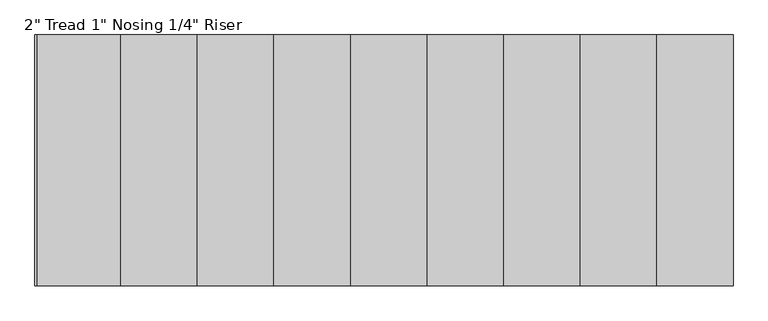
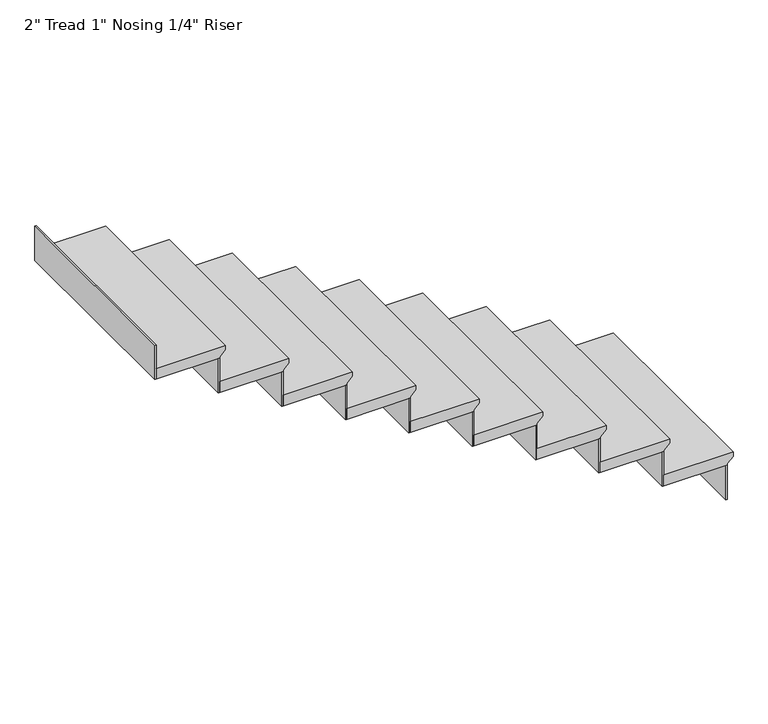
"""IFC4 building model written with IfcOpenShell, lengths in millimetres: stair flight geometry."""

from ifc_helpers import new_model, si_unit, frame, origin, place, context, project, spatial, polyline, outline, extrude, source, transform, mapped, element, save


def stair_flight_de92f90a(model_context):
    return source(origin(), model_context, "Body", "SweptSolid", [
        extrude(outline(polyline([(17762.22, 923.4845537), (17762.22, 618.6845537), (17711.42, 618.6845537), (17711.42, 898.0845537), (17717.77, 898.0845537), (17743.17, 923.4845537), (17762.22, 923.4845537)])), frame((0.0, -5753.3544725, 0.0), z_axis=(0.0, 1.0, 0.0), x_axis=(0.0, 0.0, 1.0)), (0.0, 0.0, 1.0), 914.4),
        extrude(outline(polyline([(891.7345537, -4838.9544725), (898.0845537, -4838.9544725), (898.0845537, -5753.3544725), (891.7345537, -5753.3544725), (891.7345537, -4838.9544725)])), frame((0.0, 0.0, 17551.4), z_axis=(0.0, 0.0, 1.0), x_axis=(1.0, 0.0, 0.0)), (0.0, 0.0, 1.0), 160.02),
        extrude(outline(polyline([(612.3345537, -4838.9544725), (618.6845537, -4838.9544725), (618.6845537, -5753.3544725), (612.3345537, -5753.3544725), (612.3345537, -4838.9544725)])), frame((0.0, 0.0, 17711.42), z_axis=(0.0, 0.0, 1.0), x_axis=(1.0, 0.0, 0.0)), (0.0, 0.0, 1.0), 160.02),
        extrude(outline(polyline([(17922.24, 644.0845537), (17922.24, 339.2845537), (17871.44, 339.2845537), (17871.44, 618.6845537), (17877.79, 618.6845537), (17903.19, 644.0845537), (17922.24, 644.0845537)])), frame((0.0, -5753.3544725, 0.0), z_axis=(0.0, 1.0, 0.0), x_axis=(0.0, 0.0, 1.0)), (0.0, 0.0, 1.0), 914.4),
        extrude(outline(polyline([(332.9345537, -4838.9544725), (339.2845537, -4838.9544725), (339.2845537, -5753.3544725), (332.9345537, -5753.3544725), (332.9345537, -4838.9544725)])), frame((0.0, 0.0, 17871.44), z_axis=(0.0, 0.0, 1.0), x_axis=(1.0, 0.0, 0.0)), (0.0, 0.0, 1.0), 160.02),
        extrude(outline(polyline([(18082.26, 364.6845537), (18082.26, 59.8845537), (18031.46, 59.8845537), (18031.46, 339.2845537), (18037.81, 339.2845537), (18063.21, 364.6845537), (18082.26, 364.6845537)])), frame((0.0, -5753.3544725, 0.0), z_axis=(0.0, 1.0, 0.0), x_axis=(0.0, 0.0, 1.0)), (0.0, 0.0, 1.0), 914.4),
        extrude(outline(polyline([(53.5345537, -4838.9544725), (59.8845537, -4838.9544725), (59.8845537, -5753.3544725), (53.5345537, -5753.3544725), (53.5345537, -4838.9544725)])), frame((0.0, 0.0, 18031.46), z_axis=(0.0, 0.0, 1.0), x_axis=(1.0, 0.0, 0.0)), (0.0, 0.0, 1.0), 160.02),
        extrude(outline(polyline([(18242.28, 85.2845537), (18242.28, -219.5154463), (18191.48, -219.5154463), (18191.48, 59.8845537), (18197.83, 59.8845537), (18223.23, 85.2845537), (18242.28, 85.2845537)])), frame((0.0, -5753.3544725, 0.0), z_axis=(0.0, 1.0, 0.0), x_axis=(0.0, 0.0, 1.0)), (0.0, 0.0, 1.0), 914.4),
        extrude(outline(polyline([(-225.8654463, -4838.9544725), (-219.5154463, -4838.9544725), (-219.5154463, -5753.3544725), (-225.8654463, -5753.3544725), (-225.8654463, -4838.9544725)])), frame((0.0, 0.0, 18191.48), z_axis=(0.0, 0.0, 1.0), x_axis=(1.0, 0.0, 0.0)), (0.0, 0.0, 1.0), 160.02),
        extrude(outline(polyline([(18402.3, -194.1154463), (18402.3, -498.9154463), (18351.5, -498.9154463), (18351.5, -219.5154463), (18357.85, -219.5154463), (18383.25, -194.1154463), (18402.3, -194.1154463)])), frame((0.0, -5753.3544725, 0.0), z_axis=(0.0, 1.0, 0.0), x_axis=(0.0, 0.0, 1.0)), (0.0, 0.0, 1.0), 914.4),
        extrude(outline(polyline([(-505.2654463, -4838.9544725), (-498.9154463, -4838.9544725), (-498.9154463, -5753.3544725), (-505.2654463, -5753.3544725), (-505.2654463, -4838.9544725)])), frame((0.0, 0.0, 18351.5), z_axis=(0.0, 0.0, 1.0), x_axis=(1.0, 0.0, 0.0)), (0.0, 0.0, 1.0), 160.02),
        extrude(outline(polyline([(18562.32, -473.5154463), (18562.32, -778.3154463), (18511.52, -778.3154463), (18511.52, -498.9154463), (18517.87, -498.9154463), (18543.27, -473.5154463), (18562.32, -473.5154463)])), frame((0.0, -5753.3544725, 0.0), z_axis=(0.0, 1.0, 0.0), x_axis=(0.0, 0.0, 1.0)), (0.0, 0.0, 1.0), 914.4),
        extrude(outline(polyline([(-784.6654463, -4838.9544725), (-778.3154463, -4838.9544725), (-778.3154463, -5753.3544725), (-784.6654463, -5753.3544725), (-784.6654463, -4838.9544725)])), frame((0.0, 0.0, 18511.52), z_axis=(0.0, 0.0, 1.0), x_axis=(1.0, 0.0, 0.0)), (0.0, 0.0, 1.0), 160.02),
        extrude(outline(polyline([(18722.34, -752.9154463), (18722.34, -1057.7154463), (18671.54, -1057.7154463), (18671.54, -778.3154463), (18677.89, -778.3154463), (18703.29, -752.9154463), (18722.34, -752.9154463)])), frame((0.0, -5753.3544725, 0.0), z_axis=(0.0, 1.0, 0.0), x_axis=(0.0, 0.0, 1.0)), (0.0, 0.0, 1.0), 914.4),
        extrude(outline(polyline([(-1064.0654463, -4838.9544725), (-1057.7154463, -4838.9544725), (-1057.7154463, -5753.3544725), (-1064.0654463, -5753.3544725), (-1064.0654463, -4838.9544725)])), frame((0.0, 0.0, 18671.54), z_axis=(0.0, 0.0, 1.0), x_axis=(1.0, 0.0, 0.0)), (0.0, 0.0, 1.0), 160.02),
        extrude(outline(polyline([(18882.36, -1032.3154463), (18882.36, -1337.1154463), (18831.56, -1337.1154463), (18831.56, -1057.7154463), (18837.91, -1057.7154463), (18863.31, -1032.3154463), (18882.36, -1032.3154463)])), frame((0.0, -5753.3544725, 0.0), z_axis=(0.0, 1.0, 0.0), x_axis=(0.0, 0.0, 1.0)), (0.0, 0.0, 1.0), 914.4),
        extrude(outline(polyline([(-1343.4654463, -4838.9544725), (-1337.1154463, -4838.9544725), (-1337.1154463, -5753.3544725), (-1343.4654463, -5753.3544725), (-1343.4654463, -4838.9544725)])), frame((0.0, 0.0, 18831.56), z_axis=(0.0, 0.0, 1.0), x_axis=(1.0, 0.0, 0.0)), (0.0, 0.0, 1.0), 160.02),
        extrude(outline(polyline([(-1622.8654463, -4838.9544725), (-1616.5154463, -4838.9544725), (-1616.5154463, -5753.3544725), (-1622.8654463, -5753.3544725), (-1622.8654463, -4838.9544725)])), frame((0.0, 0.0, 18991.58), z_axis=(0.0, 0.0, 1.0), x_axis=(1.0, 0.0, 0.0)), (0.0, 0.0, 1.0), 160.02),
        extrude(outline(polyline([(19042.38, -1311.7154463), (19042.38, -1616.5154463), (18991.58, -1616.5154463), (18991.58, -1337.1154463), (18997.93, -1337.1154463), (19023.33, -1311.7154463), (19042.38, -1311.7154463)])), frame((0.0, -5753.3544725, 0.0), z_axis=(0.0, 1.0, 0.0), x_axis=(0.0, 0.0, 1.0)), (0.0, 0.0, 1.0), 914.4),
    ])


if __name__ == "__main__":
    model = new_model("IFC4")
    model_context = context("Model", 3, world=origin())
    ifc_project = project(units=[si_unit("LENGTHUNIT", "METRE", prefix="MILLI")], contexts=[model_context])
    site = spatial("IfcSite", under=ifc_project)
    building = spatial("IfcBuilding", under=site)
    placement = place(None, origin())
    stair_flight_shape = stair_flight_de92f90a(model_context)
    element("IfcStairFlight", 1, ObjectType="2\" Tread 1\" Nosing 1/4\" Riser", at=placement, inside=building, context=model_context, shape_type="MappedRepresentation", body=[
        mapped(stair_flight_shape, transform((0.0, 0.0, 0.0), x_axis=(1.0, 0.0, 0.0), y_axis=(0.0, 1.0, 0.0), z_axis=(0.0, 0.0, 1.0))),
    ])
    save(model, "model.ifc")
